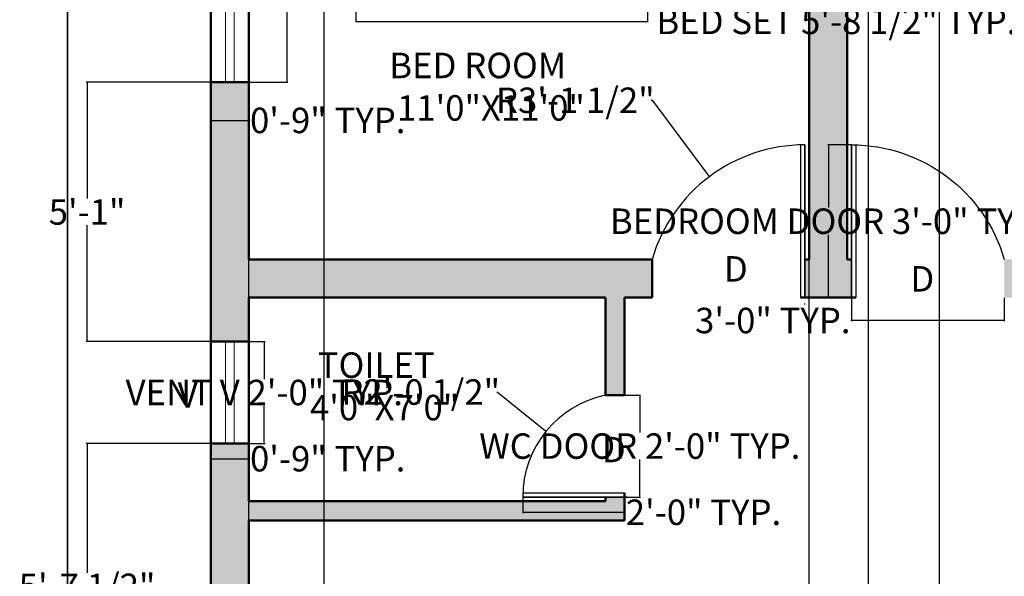
# Model space of a CAD drawing. Units: inches. Extents: x 125920 to 126336, y 366134 to 366735.
# Tile 4 of 6: x 125921 to 126153, y 366473 to 366604. Entities that reach past the tile are written whole.
import ezdxf

# ---------------------------------------------------------------- set-up
doc = ezdxf.new("R2010")
doc.units = ezdxf.units.IN
doc.header["$MEASUREMENT"] = 0
for name, color, linetype, lineweight in [('A-ANNO-DIMS', 2, 'Continuous', 18), ('A-ANNO-TEXT', 7, 'Continuous', 18), ('A-ANNO-TTLB', 7, 'Continuous', 35), ('A-AREA-IDEN', 7, 'Continuous', 25), ('A-DOOR', 3, 'Continuous', 25), ('A-GLAZ', 4, 'Continuous', 18), ('A-WALL', 7, 'Continuous', 50)]:
    doc.layers.add(name, color=color, linetype=linetype, lineweight=lineweight)
doc.layers.add('A-WALL-PATT', color=18, linetype='Continuous', lineweight=13, true_color=0x000000)
doc.styles.get("Standard").update_dxf_attribs({"font": 'arial.ttf'})
doc.dimstyles.get("Standard").update_dxf_attribs({"dimtxt": 6, "dimasz": 0.18, "dimexe": 0.18, "dimexo": 0.0625, "dimgap": 0.09, "dimtad": 0, "dimtih": 1, "dimtoh": 1, "dimdec": 1, "dimzin": 0, "dimdsep": 46, "dimlunit": 3, "dimtxsty": 'Standard', "dimcen": 0.09, "dimadec": 0, "dimazin": 0, "dimtfac": 1, "dimtdec": 1, "dimtofl": 0, "dimtmove": 0, "dimatfit": 3, "dimfxl": 1, "dimtolj": 1, "dimtzin": 0, "dimarcsym": 0})

# ---------------------------------------------------------------- blocks, each defined once
blk = doc.blocks.new('WIN-60')
for p, q in [((0, 0), (0, 60)), ((3.5, 0), (3.5, 60)), ((5.5, 60), (5.5, 0)), ((9, 60), (9, 0))]:
    blk.add_line(p, q)
blk = doc.blocks.new('VENT-24')
for p, q in [((0, 0), (0, 24)), ((3.5, 0), (3.5, 24)), ((5.5, 24), (5.5, 0)), ((9, 24), (9, 0))]:
    blk.add_line(p, q)
blk = doc.blocks.new('DOOR-36-WALL-9')
for p, q in [((35, 36), (35, 0)), ((36, 0), (36, 36)), ((36, 0), (35, 0))]:
    blk.add_line(p, q)
blk.add_arc((36, -1.5), 37.5, 90, 163.7398)
blk = doc.blocks.new('DOOR-24-WALL-4_5')
for p, q in [((0, 1), (24, 1)), ((24, 0), (24, 1)), ((24, 0), (0, 0))]:
    blk.add_line(p, q)
blk.add_arc((24.52, 0), 24.52, 101.8123, 180)
blk = doc.blocks.new('*D13')
at = {"layer": 'A-ANNO-DIMS', "color": 0, "lineweight": -2, "transparency": 16777216}
for p, q in [((125975.54, 366649.55), (125984.65, 366649.55)), ((125984.47, 366649.37), (125984.47, 366622.75)), ((125984.47, 366589.73), (125984.47, 366616.36)), ((125975.54, 366589.55), (125984.65, 366589.55))]:
    blk.add_line(p, q, dxfattribs=at)
at = {"layer": 'A-ANNO-DIMS', "color": 0, "transparency": 16777216}
for points in [[(125984.44, 366649.37), (125984.5, 366649.37), (125984.47, 366649.55)], [(125984.44, 366589.73), (125984.5, 366589.73), (125984.47, 366589.55)]]:
    blk.add_solid(points, dxfattribs=at)
at = {"layer": 'Defpoints', "color": 0, "transparency": 16777216}
for p in [(125975.47, 366649.55), (125984.47, 366649.55), (125975.47, 366589.55)]:
    blk.add_point(p, dxfattribs=at)
at = {"layer": 'A-ANNO-DIMS', "color": 0, "transparency": 16777216, "insert": (125984.47, 366619.55), "char_height": 6, "attachment_point": 5}
blk.add_mtext('\\A1;WINDOW W 5\'-0" TYP.', dxfattribs=at)
blk = doc.blocks.new('*D14')
at = {"layer": 'A-ANNO-DIMS', "color": 0, "lineweight": -2, "transparency": 16777216}
for p, q in [((125966.47, 366589.49), (125966.47, 366580.37)), ((125975.47, 366589.49), (125975.47, 366580.37)), ((125966.65, 366580.55), (125975.29, 366580.55)), ((125975.47, 366580.55), (125975.65, 366580.55))]:
    blk.add_line(p, q, dxfattribs=at)
at = {"layer": 'A-ANNO-DIMS', "color": 0, "transparency": 16777216}
for points in [[(125966.65, 366580.58), (125966.65, 366580.52), (125966.47, 366580.55)], [(125975.29, 366580.58), (125975.29, 366580.52), (125975.47, 366580.55)]]:
    blk.add_solid(points, dxfattribs=at)
at = {"layer": 'Defpoints', "color": 0, "transparency": 16777216}
for p in [(125966.47, 366589.55), (125975.47, 366589.55), (125975.47, 366580.55)]:
    blk.add_point(p, dxfattribs=at)
at = {"layer": 'A-ANNO-DIMS', "color": 0, "transparency": 16777216, "insert": (125994.03, 366580.55), "char_height": 6, "attachment_point": 5}
blk.add_mtext('\\A1;0\'-9" TYP.', dxfattribs=at)
blk = doc.blocks.new('*D17')
at = {"layer": 'A-ANNO-DIMS', "color": 0, "lineweight": -2, "transparency": 16777216}
for p, q in [((125975.54, 366528.42), (125979.25, 366528.42)), ((125979.07, 366528.24), (125979.07, 366519.57)), ((125979.07, 366504.6), (125979.07, 366513.26)), ((125975.54, 366504.42), (125979.25, 366504.42))]:
    blk.add_line(p, q, dxfattribs=at)
at = {"layer": 'A-ANNO-DIMS', "color": 0, "transparency": 16777216}
for points in [[(125979.04, 366528.24), (125979.1, 366528.24), (125979.07, 366528.42)], [(125979.04, 366504.6), (125979.1, 366504.6), (125979.07, 366504.42)]]:
    blk.add_solid(points, dxfattribs=at)
at = {"layer": 'Defpoints', "color": 0, "transparency": 16777216}
for p in [(125975.47, 366528.42), (125979.07, 366528.42), (125975.47, 366504.42)]:
    blk.add_point(p, dxfattribs=at)
at = {"layer": 'A-ANNO-DIMS', "color": 0, "transparency": 16777216, "insert": (125979.07, 366516.42), "char_height": 6, "attachment_point": 5}
blk.add_mtext('\\A1;VENT V 2\'-0" TYP.', dxfattribs=at)
blk = doc.blocks.new('*D18')
at = {"layer": 'A-ANNO-DIMS', "color": 0, "lineweight": -2, "transparency": 16777216}
for p, q in [((125966.47, 366504.35), (125966.47, 366500.64)), ((125975.47, 366504.35), (125975.47, 366500.64)), ((125966.65, 366500.82), (125975.29, 366500.82)), ((125975.47, 366500.82), (125975.65, 366500.82))]:
    blk.add_line(p, q, dxfattribs=at)
at = {"layer": 'A-ANNO-DIMS', "color": 0, "transparency": 16777216}
for points in [[(125966.65, 366500.85), (125966.65, 366500.79), (125966.47, 366500.82)], [(125975.29, 366500.85), (125975.29, 366500.79), (125975.47, 366500.82)]]:
    blk.add_solid(points, dxfattribs=at)
at = {"layer": 'Defpoints', "color": 0, "transparency": 16777216}
for p in [(125966.47, 366504.42), (125975.47, 366504.42), (125975.47, 366500.82)]:
    blk.add_point(p, dxfattribs=at)
at = {"layer": 'A-ANNO-DIMS', "color": 0, "transparency": 16777216, "insert": (125994.03, 366500.82), "char_height": 6, "attachment_point": 5}
blk.add_mtext('\\A1;0\'-9" TYP.', dxfattribs=at)
blk = doc.blocks.new('*D19')
at = {"layer": 'A-ANNO-DIMS', "color": 0, "lineweight": -2, "transparency": 16777216}
for p, q in [((126000.69, 366614.13), (126000.69, 366603.71)), ((126069.4, 366614.13), (126069.4, 366603.71)), ((126000.87, 366603.89), (126069.22, 366603.89)), ((126069.4, 366603.89), (126069.58, 366603.89))]:
    blk.add_line(p, q, dxfattribs=at)
at = {"layer": 'A-ANNO-DIMS', "color": 0, "transparency": 16777216}
for points in [[(126000.87, 366603.92), (126000.87, 366603.86), (126000.69, 366603.89)], [(126069.22, 366603.92), (126069.22, 366603.86), (126069.4, 366603.89)]]:
    blk.add_solid(points, dxfattribs=at)
at = {"layer": 'Defpoints', "color": 0, "transparency": 16777216}
for p in [(126000.69, 366614.19), (126069.4, 366614.19), (126069.4, 366603.89)]:
    blk.add_point(p, dxfattribs=at)
at = {"layer": 'A-ANNO-DIMS', "color": 0, "transparency": 16777216, "insert": (126113.91, 366603.89), "char_height": 6, "attachment_point": 5}
blk.add_mtext('\\A1;BED SET 5\'-8 1/2" TYP.', dxfattribs=at)
blk = doc.blocks.new('*D25')
at = {"layer": 'A-ANNO-DIMS', "color": 0, "lineweight": -2, "transparency": 16777216}
for p, q in [((126117.41, 366574.79), (126111.89, 366574.79)), ((126112.07, 366574.61), (126112.07, 366559.99)), ((126112.07, 366538.97), (126112.07, 366553.6)), ((126117.41, 366538.79), (126111.89, 366538.79))]:
    blk.add_line(p, q, dxfattribs=at)
at = {"layer": 'A-ANNO-DIMS', "color": 0, "transparency": 16777216}
for points in [[(126112.04, 366574.61), (126112.1, 366574.61), (126112.07, 366574.79)], [(126112.04, 366538.97), (126112.1, 366538.97), (126112.07, 366538.79)]]:
    blk.add_solid(points, dxfattribs=at)
at = {"layer": 'Defpoints', "color": 0, "transparency": 16777216}
for p in [(126112.07, 366574.79), (126117.47, 366574.79), (126117.47, 366538.79)]:
    blk.add_point(p, dxfattribs=at)
at = {"layer": 'A-ANNO-DIMS', "color": 0, "transparency": 16777216, "insert": (126112.07, 366556.79), "char_height": 6, "attachment_point": 5}
blk.add_mtext('\\A1;BEDROOM DOOR 3\'-0" TYP.', dxfattribs=at)
blk = doc.blocks.new('*D26')
at = {"layer": 'A-ANNO-DIMS', "color": 0, "lineweight": -2, "transparency": 16777216}
for p, q in [((126117.47, 366538.73), (126117.47, 366533.21)), ((126153.47, 366538.73), (126153.47, 366533.21)), ((126117.47, 366533.39), (126117.29, 366533.39)), ((126153.29, 366533.39), (126117.65, 366533.39))]:
    blk.add_line(p, q, dxfattribs=at)
at = {"layer": 'A-ANNO-DIMS', "color": 0, "transparency": 16777216}
for points in [[(126117.65, 366533.42), (126117.65, 366533.36), (126117.47, 366533.39)], [(126153.29, 366533.42), (126153.29, 366533.36), (126153.47, 366533.39)]]:
    blk.add_solid(points, dxfattribs=at)
at = {"layer": 'Defpoints', "color": 0, "transparency": 16777216}
for p in [(126117.47, 366538.79), (126153.47, 366538.79), (126117.47, 366533.39)]:
    blk.add_point(p, dxfattribs=at)
at = {"layer": 'A-ANNO-DIMS', "color": 0, "transparency": 16777216, "insert": (126098.92, 366533.39), "char_height": 6, "attachment_point": 5}
blk.add_mtext('\\A1;3\'-0" TYP.', dxfattribs=at)
blk = doc.blocks.new('*D27')
at = {"layer": 'A-ANNO-DIMS', "color": 0, "lineweight": -2, "transparency": 16777216}
for p, q in [((126064.04, 366515.79), (126067.75, 366515.79)), ((126067.57, 366515.61), (126067.57, 366506.99)), ((126067.57, 366491.97), (126067.57, 366500.6)), ((126064.04, 366491.79), (126067.75, 366491.79))]:
    blk.add_line(p, q, dxfattribs=at)
at = {"layer": 'A-ANNO-DIMS', "color": 0, "transparency": 16777216}
for points in [[(126067.54, 366515.61), (126067.6, 366515.61), (126067.57, 366515.79)], [(126067.54, 366491.97), (126067.6, 366491.97), (126067.57, 366491.79)]]:
    blk.add_solid(points, dxfattribs=at)
at = {"layer": 'Defpoints', "color": 0, "transparency": 16777216}
for p in [(126063.97, 366515.79), (126067.57, 366515.79), (126063.97, 366491.79)]:
    blk.add_point(p, dxfattribs=at)
at = {"layer": 'A-ANNO-DIMS', "color": 0, "transparency": 16777216, "insert": (126067.57, 366503.79), "char_height": 6, "attachment_point": 5}
blk.add_mtext('\\A1;WC DOOR 2\'-0" TYP.', dxfattribs=at)
blk = doc.blocks.new('*D28')
at = {"layer": 'A-ANNO-DIMS', "color": 0, "lineweight": -2, "transparency": 16777216}
for p, q in [((126039.97, 366491.73), (126039.97, 366488.01)), ((126063.97, 366491.73), (126063.97, 366488.01)), ((126040.15, 366488.19), (126063.79, 366488.19)), ((126063.97, 366488.19), (126064.15, 366488.19))]:
    blk.add_line(p, q, dxfattribs=at)
at = {"layer": 'A-ANNO-DIMS', "color": 0, "transparency": 16777216}
for points in [[(126040.15, 366488.22), (126040.15, 366488.16), (126039.97, 366488.19)], [(126063.79, 366488.22), (126063.79, 366488.16), (126063.97, 366488.19)]]:
    blk.add_solid(points, dxfattribs=at)
at = {"layer": 'Defpoints', "color": 0, "transparency": 16777216}
for p in [(126039.97, 366491.79), (126063.97, 366491.79), (126063.97, 366488.19)]:
    blk.add_point(p, dxfattribs=at)
at = {"layer": 'A-ANNO-DIMS', "color": 0, "transparency": 16777216, "insert": (126082.58, 366488.19), "char_height": 6, "attachment_point": 5}
blk.add_mtext('\\A1;2\'-0" TYP.', dxfattribs=at)
blk = doc.blocks.new('*D30')
at = {"layer": 'A-ANNO-DIMS', "color": 0, "lineweight": -2, "transparency": 16777216}
for p, q in [((125966.41, 366504.42), (125937.14, 366504.42)), ((125937.32, 366504.24), (125937.32, 366473.94)), ((125937.32, 366437.25), (125937.32, 366467.55)), ((125966.41, 366437.07), (125937.14, 366437.07))]:
    blk.add_line(p, q, dxfattribs=at)
at = {"layer": 'A-ANNO-DIMS', "color": 0, "transparency": 16777216}
for points in [[(125937.29, 366504.24), (125937.35, 366504.24), (125937.32, 366504.42)], [(125937.29, 366437.25), (125937.35, 366437.25), (125937.32, 366437.07)]]:
    blk.add_solid(points, dxfattribs=at)
at = {"layer": 'Defpoints', "color": 0, "transparency": 16777216}
for p in [(125937.32, 366504.42), (125966.47, 366504.42), (125966.47, 366437.07)]:
    blk.add_point(p, dxfattribs=at)
at = {"layer": 'A-ANNO-DIMS', "color": 0, "transparency": 16777216, "insert": (125937.32, 366470.74), "char_height": 6, "attachment_point": 5}
blk.add_mtext('\\A1;5\'-7 1/2"', dxfattribs=at)
blk = doc.blocks.new('*D31')
at = {"layer": 'A-ANNO-DIMS', "color": 0, "lineweight": -2, "transparency": 16777216}
for p, q in [((125966.41, 366589.55), (125937.14, 366589.55)), ((125937.32, 366589.37), (125937.32, 366562.14)), ((125937.32, 366528.6), (125937.32, 366555.83)), ((125966.41, 366528.42), (125937.14, 366528.42))]:
    blk.add_line(p, q, dxfattribs=at)
at = {"layer": 'A-ANNO-DIMS', "color": 0, "transparency": 16777216}
for points in [[(125937.29, 366589.37), (125937.35, 366589.37), (125937.32, 366589.55)], [(125937.29, 366528.6), (125937.35, 366528.6), (125937.32, 366528.42)]]:
    blk.add_solid(points, dxfattribs=at)
at = {"layer": 'Defpoints', "color": 0, "transparency": 16777216}
for p in [(125937.32, 366589.55), (125966.47, 366589.55), (125966.47, 366528.42)]:
    blk.add_point(p, dxfattribs=at)
at = {"layer": 'A-ANNO-DIMS', "color": 0, "transparency": 16777216, "insert": (125937.32, 366558.98), "char_height": 6, "attachment_point": 5}
blk.add_mtext('\\A1;5\'-1"', dxfattribs=at)
blk = doc.blocks.new('*D40')
at = {"layer": 'A-ANNO-DIMS', "color": 0, "lineweight": -2, "transparency": 16777216}
for p, q in [((126107.47, 366288.86), (126107.47, 366718.12)), ((126107.65, 366717.94), (126114.73, 366717.94)), ((126138.05, 366717.94), (126130.97, 366717.94)), ((126138.23, 366288.86), (126138.23, 366718.12))]:
    blk.add_line(p, q, dxfattribs=at)
at = {"layer": 'A-ANNO-DIMS', "color": 0, "transparency": 16777216}
for points in [[(126107.65, 366717.97), (126107.65, 366717.91), (126107.47, 366717.94)], [(126138.05, 366717.97), (126138.05, 366717.91), (126138.23, 366717.94)]]:
    blk.add_solid(points, dxfattribs=at)
at = {"layer": 'Defpoints', "color": 0, "transparency": 16777216}
for p in [(126138.23, 366717.94), (126107.47, 366288.79), (126138.23, 366288.79)]:
    blk.add_point(p, dxfattribs=at)
at = {"layer": 'A-ANNO-DIMS', "color": 0, "transparency": 16777216, "insert": (126122.85, 366717.94), "char_height": 6, "attachment_point": 5}
blk.add_mtext('\\A1;2\'-7"', dxfattribs=at)
blk = doc.blocks.new('*D41')
at = {"layer": 'A-ANNO-DIMS', "color": 0, "lineweight": -2, "transparency": 16777216}
for p, q in [((126121.47, 366216.86), (126121.47, 366718.12)), ((126121.65, 366717.94), (126163.4, 366717.94)), ((126221.29, 366717.94), (126179.54, 366717.94)), ((126221.47, 366216.86), (126221.47, 366718.12))]:
    blk.add_line(p, q, dxfattribs=at)
at = {"layer": 'A-ANNO-DIMS', "color": 0, "transparency": 16777216}
for points in [[(126121.65, 366717.97), (126121.65, 366717.91), (126121.47, 366717.94)], [(126221.29, 366717.97), (126221.29, 366717.91), (126221.47, 366717.94)]]:
    blk.add_solid(points, dxfattribs=at)
at = {"layer": 'Defpoints', "color": 0, "transparency": 16777216}
for p in [(126221.47, 366717.94), (126121.47, 366216.79), (126221.47, 366216.79)]:
    blk.add_point(p, dxfattribs=at)
at = {"layer": 'A-ANNO-DIMS', "color": 0, "transparency": 16777216, "insert": (126171.47, 366717.94), "char_height": 6, "attachment_point": 5}
blk.add_mtext('\\A1;8\'-4"', dxfattribs=at)
blk = doc.blocks.new('*D45')
at = {"layer": 'A-ANNO-DIMS', "color": 0, "lineweight": -2, "transparency": 16777216}
for p, q in [((125975.47, 366216.86), (125975.47, 366718.12)), ((125975.65, 366717.94), (125992.98, 366717.94)), ((125993.16, 366235.36), (125993.16, 366718.12)), ((125993.16, 366717.94), (125993.34, 366717.94))]:
    blk.add_line(p, q, dxfattribs=at)
at = {"layer": 'A-ANNO-DIMS', "color": 0, "transparency": 16777216}
for points in [[(125975.65, 366717.97), (125975.65, 366717.91), (125975.47, 366717.94)], [(125992.98, 366717.97), (125992.98, 366717.91), (125993.16, 366717.94)]]:
    blk.add_solid(points, dxfattribs=at)
at = {"layer": 'Defpoints', "color": 0, "transparency": 16777216}
for p in [(125993.16, 366717.94), (125993.16, 366235.3), (125975.47, 366216.79)]:
    blk.add_point(p, dxfattribs=at)
at = {"layer": 'A-ANNO-DIMS', "color": 0, "transparency": 16777216, "insert": (126008.11, 366717.94), "char_height": 6, "attachment_point": 5}
blk.add_mtext('\\A1;1\'-5 1/2"', dxfattribs=at)
blk = doc.blocks.new('*D48')
at = {"layer": 'A-ANNO-DIMS', "color": 0, "lineweight": -2, "transparency": 16777216}
for p, q in [((126070.29, 366585.29), (126070.47, 366585.29)), ((126070.47, 366585.29), (126083.87, 366567.44)), ((126106.38, 366537.29), (126106.56, 366537.29)), ((126106.47, 366537.2), (126106.47, 366537.38))]:
    blk.add_line(p, q, dxfattribs=at)
at = {"layer": 'A-ANNO-DIMS', "color": 0, "transparency": 16777216}
blk.add_solid([(126083.89, 366567.46), (126083.84, 366567.42), (126083.97, 366567.29)], dxfattribs=at)
at = {"layer": 'Defpoints', "color": 0, "transparency": 16777216}
for p in [(126083.97, 366567.29), (126106.47, 366537.29)]:
    blk.add_point(p, dxfattribs=at)
at = {"layer": 'A-ANNO-DIMS', "color": 0, "transparency": 16777216, "insert": (126052.37, 366585.29), "char_height": 6, "attachment_point": 5}
blk.add_mtext('\\A1;R3\'-1 1/2"', dxfattribs=at)
blk = doc.blocks.new('*D51')
at = {"layer": 'A-ANNO-DIMS', "color": 0, "lineweight": -2, "transparency": 16777216}
for p, q in [((126033.86, 366516.53), (126034.04, 366516.53)), ((126034.04, 366516.53), (126045.32, 366507.37)), ((126064.4, 366491.79), (126064.58, 366491.79)), ((126064.49, 366491.7), (126064.49, 366491.88))]:
    blk.add_line(p, q, dxfattribs=at)
at = {"layer": 'A-ANNO-DIMS', "color": 0, "transparency": 16777216}
blk.add_solid([(126045.34, 366507.39), (126045.3, 366507.35), (126045.46, 366507.26)], dxfattribs=at)
at = {"layer": 'Defpoints', "color": 0, "transparency": 16777216}
for p in [(126045.46, 366507.26), (126064.49, 366491.79)]:
    blk.add_point(p, dxfattribs=at)
at = {"layer": 'A-ANNO-DIMS', "color": 0, "transparency": 16777216, "insert": (126015.94, 366516.53), "char_height": 6, "attachment_point": 5}
blk.add_mtext('\\A1;R2\'-0 1/2"', dxfattribs=at)

msp = doc.modelspace()

# ---------------------------------------------------------------- hatches: boundary and pattern name
at = {"layer": 'A-WALL-PATT'}
h = msp.add_hatch(color=256, dxfattribs=at)
h.dxf.hatch_style = 1
h.paths.add_polyline_path([(126266.47, 366688.79), (125966.47, 366688.79), (125966.47, 366649.55), (125975.47, 366649.55), (125975.47, 366679.79), (126107.47, 366679.79), (126107.47, 366547.79), (126106.47, 366547.79), (126106.47, 366538.79), (126107.47, 366538.79), (126117.47, 366538.79), (126117.47, 366547.79), (126116.47, 366547.79), (126116.47, 366679.79), (126257.47, 366679.79), (126257.47, 366648.33), (126266.47, 366648.33)])
h.paths.add_polyline_path([(126070.47, 366547.79), (125975.47, 366547.79), (125975.47, 366589.55), (125966.47, 366589.55), (125966.47, 366528.42), (125975.47, 366528.42), (125975.47, 366538.79), (126059.47, 366538.79), (126059.47, 366515.79), (126063.97, 366515.79), (126063.97, 366538.79), (126070.47, 366538.79)])
h.paths.add_polyline_path([(125975.47, 366486.29), (126063.97, 366486.29), (126063.97, 366491.79), (126059.47, 366491.79), (126059.47, 366490.79), (125975.47, 366490.79), (125975.47, 366504.42), (125966.47, 366504.42), (125966.47, 366437.07), (125975.47, 366437.07)])
h.paths.add_polyline_path([(125975.47, 366312.79), (126022.47, 366312.79), (126022.47, 366317.29), (125975.47, 366317.29), (125975.47, 366377.07), (125966.47, 366377.07), (125966.47, 366207.79), (125987.64, 366207.79), (125987.64, 366216.79), (125975.47, 366216.79)])
h.paths.add_polyline_path([(126063.97, 366216.79), (126063.97, 366312.79), (126070.47, 366312.79), (126070.47, 366317.29), (126058.47, 366317.29), (126058.47, 366312.79), (126059.47, 366312.79), (126059.47, 366216.79), (126047.64, 366216.79), (126047.64, 366207.79), (126063.97, 366207.79)])
h.paths.add_polyline_path([(126221.47, 366216.79), (126116.47, 366216.79), (126107.47, 366216.79), (126107.47, 366207.79), (126221.47, 366207.79)])
h.paths.add_polyline_path([(126266.47, 366336.48), (126257.47, 366336.48), (126257.47, 366297.79), (126174.23, 366297.79), (126174.23, 366288.79), (126257.47, 366288.79), (126257.47, 366207.79), (126266.47, 366207.79)])
h.paths.add_polyline_path([(126138.23, 366297.79), (126116.47, 366297.79), (126116.47, 366433.79), (126117.47, 366433.79), (126117.47, 366438.29), (126116.47, 366438.29), (126107.47, 366438.29), (126107.47, 366317.29), (126106.47, 366317.29), (126106.47, 366312.79), (126107.47, 366312.79), (126107.47, 366288.79), (126116.47, 366288.79), (126138.23, 366288.79)])
h.paths.add_polyline_path([(126266.47, 366449.1), (126257.47, 366449.1), (126257.47, 366438.29), (126256.47, 366438.29), (126256.47, 366433.79), (126257.47, 366433.79), (126257.47, 366396.48), (126266.47, 366396.48)])
h.paths.add_polyline_path([(126232.47, 366438.29), (126180.47, 366438.29), (126180.47, 366486.29), (126257.47, 366486.29), (126257.47, 366473.1), (126266.47, 366473.1), (126266.47, 366504.78), (126257.47, 366504.78), (126257.47, 366490.79), (126180.47, 366490.79), (126180.47, 366538.79), (126232.47, 366538.79), (126232.47, 366547.79), (126153.47, 366547.79), (126153.47, 366538.79), (126175.97, 366538.79), (126175.97, 366438.29), (126153.47, 366438.29), (126153.47, 366433.79), (126232.47, 366433.79)])
h.paths.add_polyline_path([(126266.47, 366588.33), (126257.47, 366588.33), (126257.47, 366547.79), (126256.47, 366547.79), (126256.47, 366538.79), (126257.47, 366538.79), (126257.47, 366528.78), (126266.47, 366528.78)])

# ---------------------------------------------------------------- linework, layer by layer
at = {"layer": 'A-ANNO-TTLB'}
msp.add_lwpolyline([(125932.73, 366735.48), (126336.24, 366735.48), (126336.24, 366133.52), (125932.73, 366133.52)], close=True, dxfattribs=at)
at = {"layer": 'A-DOOR'}
for p, q in [((126106.47, 366574.79), (126106.47, 366538.79)), ((126117.47, 366574.79), (126117.47, 366538.79)), ((126107.47, 366538.79), (126106.47, 366538.79)), ((126116.47, 366538.79), (126117.47, 366538.79)), ((126039.97, 366491.79), (126063.97, 366491.79)), ((126063.97, 366490.79), (126063.97, 366491.79))]:
    msp.add_line(p, q, dxfattribs=at)
at = {"layer": 'A-WALL'}
for p, q in [((125966.47, 366688.79), (125966.47, 366207.79)), ((125975.47, 366679.79), (125975.47, 366547.79)), ((126107.47, 366679.79), (126107.47, 366547.79)), ((126107.47, 366679.79), (126107.47, 366547.79)), ((126116.47, 366679.79), (126116.47, 366547.79)), ((126116.47, 366679.79), (126116.47, 366547.79)), ((125975.47, 366589.55), (125966.47, 366589.55)), ((125975.47, 366547.79), (126070.47, 366547.79)), ((126070.47, 366538.79), (126070.47, 366547.79)), ((126106.47, 366547.79), (126107.47, 366547.79)), ((126116.47, 366547.79), (126117.47, 366547.79)), ((125975.47, 366538.79), (126059.47, 366538.79)), ((125975.47, 366538.79), (125975.47, 366490.79)), ((126059.47, 366538.79), (126059.47, 366515.79)), ((126063.97, 366538.79), (126063.97, 366515.79)), ((126063.97, 366538.79), (126070.47, 366538.79)), ((126105.47, 366538.79), (126118.47, 366538.79)), ((125966.47, 366528.42), (125975.47, 366528.42)), ((126063.97, 366515.79), (126059.47, 366515.79)), ((125975.47, 366504.42), (125966.47, 366504.42)), ((126059.47, 366491.79), (126059.47, 366490.79)), ((126063.97, 366492.79), (126063.97, 366486.29)), ((125975.47, 366490.79), (126059.47, 366490.79)), ((125975.47, 366486.29), (126063.97, 366486.29)), ((125975.47, 366486.29), (125975.47, 366317.29))]:
    msp.add_line(p, q, dxfattribs=at)

# ---------------------------------------------------------------- block references
at = {"layer": 'A-DOOR'}
for name, p in [('DOOR-36-WALL-9', (126070.47, 366538.79)), ('DOOR-24-WALL-4_5', (126039.97, 366491.79))]:
    msp.add_blockref(name, p, dxfattribs=at)
at = {"layer": 'A-DOOR', "extrusion": (0, 0, -1), "zscale": -1}
msp.add_blockref('DOOR-36-WALL-9', (-126153.47, 366538.79), dxfattribs=at)
at = {"layer": 'A-GLAZ'}
for name, p in [('WIN-60', (125966.47, 366589.55)), ('VENT-24', (125966.47, 366504.42))]:
    msp.add_blockref(name, p, dxfattribs=at)

# ---------------------------------------------------------------- texts
at = {"layer": 'A-ANNO-TEXT', "char_height": 6, "attachment_point": 1}
for s, width, insert in [('D', 9.6923, (126087.38, 366548.56)), ('D', 9.6923, (126131.33, 366546.21)), ('V', 9.8961, (125958.67, 366518.82)), ('D', 9.6923, (126058.64, 366505.98))]:
    msp.add_mtext_dynamic_manual_height_columns(s, width=width, gutter_width=30, heights=[0], dxfattribs=dict(at, insert=insert))
at = {"layer": 'A-AREA-IDEN', "char_height": 6, "attachment_point": 1}
for s, width, insert in [('BED ROOM\\P 11\'0"X11\'0"', 54.698, (126008.53, 366596.5)), (' TOILET\\P4\'0"X7\'0"', 43.5871, (125989.85, 366525.87))]:
    msp.add_mtext_dynamic_manual_height_columns(s, width=width, gutter_width=30, heights=[0], dxfattribs=dict(at, insert=insert))

# ---------------------------------------------------------------- dimensions: what is measured, and where the dimension line sits
at = {"layer": 'A-ANNO-DIMS'}
for base, p1, p2, picture, middle in [((125993.16, 366717.94), (125975.47, 366216.79), (125993.16, 366235.3), '*D45', (126008.11, 366717.94)), ((126138.23, 366717.94), (126107.47, 366288.79), (126138.23, 366288.79), '*D40', (126122.85, 366717.94)), ((126221.47, 366717.94), (126121.47, 366216.79), (126221.47, 366216.79), '*D41', (126171.47, 366717.94))]:
    dim = msp.add_linear_dim(base=base, p1=p1, p2=p2, dimstyle='Standard', override={"dimdec": 1, "dimlfac": 1, "dimrnd": 0, "dimzin": 1, "dimdsep": 46, "dimlunit": 4, "dimfrac": 2}, dxfattribs=at)
    dim.commit()
    dim.dimension.update_dxf_attribs({"geometry": picture, "text_midpoint": middle})
for base, p1, p2, angle, text, picture, middle in [((125984.47, 366649.55), (125975.47, 366589.55), (125975.47, 366649.55), 90, 'WINDOW W <> TYP.', '*D13', (125984.47, 366619.55)), ((126112.07, 366574.79), (126117.47, 366538.79), (126117.47, 366574.79), 90, 'BEDROOM DOOR <> TYP.', '*D25', (126112.07, 366556.79)), ((126117.47, 366533.39), (126153.47, 366538.79), (126117.47, 366538.79), 180, '<> TYP.', '*D26', (126098.92, 366533.39)), ((125979.07, 366528.42), (125975.47, 366504.42), (125975.47, 366528.42), 90, 'VENT V <> TYP.', '*D17', (125979.07, 366516.42)), ((126067.57, 366515.79), (126063.97, 366491.79), (126063.97, 366515.79), 90, 'WC DOOR <> TYP.', '*D27', (126067.57, 366503.79))]:
    dim = msp.add_linear_dim(base=base, p1=p1, p2=p2, angle=angle, text=text, dimstyle='Standard', override={"dimdec": 1, "dimlfac": 1, "dimrnd": 0, "dimzin": 1, "dimdsep": 46, "dimlunit": 4, "dimfrac": 2}, dxfattribs=at)
    dim.commit()
    dim.dimension.update_dxf_attribs({"geometry": picture, "text_midpoint": middle})
for base, p1, p2, text, picture, middle in [((126069.4, 366603.89), (126000.69, 366614.19), (126069.4, 366614.19), 'BED SET <> TYP.', '*D19', (126113.91, 366603.89)), ((125975.47, 366580.55), (125966.47, 366589.55), (125975.47, 366589.55), '<> TYP.', '*D14', (125994.03, 366580.55)), ((125975.47, 366500.82), (125966.47, 366504.42), (125975.47, 366504.42), '<> TYP.', '*D18', (125994.03, 366500.82)), ((126063.97, 366488.19), (126039.97, 366491.79), (126063.97, 366491.79), '<> TYP.', '*D28', (126082.58, 366488.19))]:
    dim = msp.add_linear_dim(base=base, p1=p1, p2=p2, text=text, dimstyle='Standard', override={"dimdec": 1, "dimlfac": 1, "dimrnd": 0, "dimzin": 1, "dimdsep": 46, "dimlunit": 4, "dimfrac": 2}, dxfattribs=at)
    dim.commit()
    dim.dimension.update_dxf_attribs({"geometry": picture, "text_midpoint": middle})
for center, mpoint, picture, middle in [((126106.47, 366537.29), (126083.97, 366567.29), '*D48', (126052.37, 366585.29)), ((126064.49, 366491.79), (126045.46, 366507.26), '*D51', (126015.94, 366516.53))]:
    dim = msp.add_radius_dim(center=center, mpoint=mpoint, dimstyle='Standard', override={"dimdec": 1, "dimlfac": 1, "dimrnd": 0, "dimzin": 1, "dimdsep": 46, "dimlunit": 4, "dimfrac": 2}, dxfattribs=at)
    dim.commit()
    dim.dimension.update_dxf_attribs({"geometry": picture, "text_midpoint": middle, "dimtype": 164})
for base, p1, p2, picture, middle in [((125937.32, 366589.55), (125966.47, 366528.42), (125966.47, 366589.55), '*D31', (125937.32, 366558.98)), ((125937.3231, 366504.4154), (125966.4731, 366437.0722), (125966.4731, 366504.4154), '*D30', (125937.3231, 366470.7438))]:
    dim = msp.add_linear_dim(base=base, p1=p1, p2=p2, angle=90, dimstyle='Standard', override={"dimdec": 1, "dimlfac": 1, "dimrnd": 0, "dimzin": 1, "dimdsep": 46, "dimlunit": 4, "dimfrac": 2}, dxfattribs=at)
    dim.commit()
    dim.dimension.update_dxf_attribs({"geometry": picture, "text_midpoint": middle})

doc.saveas('drawing.dxf')
